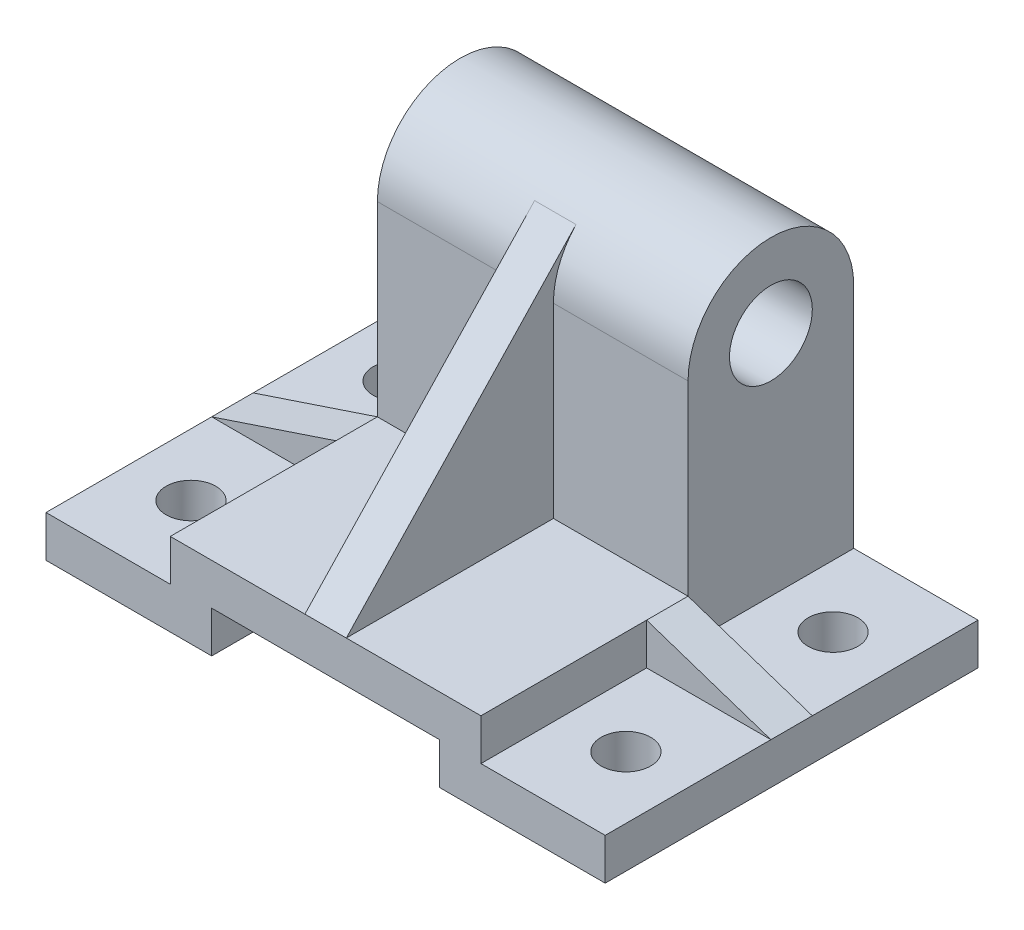
ISO-10303-21;
HEADER;
FILE_DESCRIPTION(('STEP AP214'),'2;1');
FILE_NAME('part.step','',(''),(''),'','','');
FILE_SCHEMA(('AUTOMOTIVE_DESIGN { 1 0 10303 214 1 1 1 1 }'));
ENDSEC;
DATA;
#1=APPLICATION_CONTEXT('core data for automotive mechanical design processes');
#2=APPLICATION_PROTOCOL_DEFINITION('international standard','automotive_design',2000,#1);
#3=PRODUCT_CONTEXT('',#1,'mechanical');
#4=PRODUCT('Part','Part','',(#3));
#5=PRODUCT_RELATED_PRODUCT_CATEGORY('part','',(#4));
#6=PRODUCT_DEFINITION_FORMATION('','',#4);
#7=PRODUCT_DEFINITION_CONTEXT('part definition',#1,'design');
#8=PRODUCT_DEFINITION('design','',#6,#7);
#9=PRODUCT_DEFINITION_SHAPE('','',#8);
#10=(LENGTH_UNIT() NAMED_UNIT(*) SI_UNIT(.MILLI.,.METRE.));
#11=(NAMED_UNIT(*) PLANE_ANGLE_UNIT() SI_UNIT($,.RADIAN.));
#12=(NAMED_UNIT(*) SI_UNIT($,.STERADIAN.) SOLID_ANGLE_UNIT());
#13=UNCERTAINTY_MEASURE_WITH_UNIT(LENGTH_MEASURE(1.E-05),#10,'distance_accuracy_value','');
#14=(GEOMETRIC_REPRESENTATION_CONTEXT(3) GLOBAL_UNCERTAINTY_ASSIGNED_CONTEXT((#13)) GLOBAL_UNIT_ASSIGNED_CONTEXT((#10,
#11,#12)) REPRESENTATION_CONTEXT('',''));
#15=CARTESIAN_POINT('',(0.,0.,0.));
#16=DIRECTION('',(0.,0.,1.));
#17=DIRECTION('',(1.,0.,0.));
#18=AXIS2_PLACEMENT_3D('',#15,#16,#17);
#19=CARTESIAN_POINT('',(67.5,10.,45.));
#20=DIRECTION('',(0.,-1.,0.));
#21=DIRECTION('',(1.,0.,0.));
#22=AXIS2_PLACEMENT_3D('',#19,#20,#21);
#23=PLANE('',#22);
#24=CARTESIAN_POINT('',(52.5,10.,-25.));
#25=DIRECTION('',(0.,1.,0.));
#26=DIRECTION('',(-1.,0.,0.));
#27=AXIS2_PLACEMENT_3D('',#24,#25,#26);
#28=CIRCLE('',#27,5.99999999999999);
#29=CARTESIAN_POINT('',(46.5,10.,-25.));
#30=VERTEX_POINT('',#29);
#31=EDGE_CURVE('E308',#30,#30,#28,.T.);
#32=ORIENTED_EDGE('',*,*,#31,.F.);
#33=EDGE_LOOP('',(#32));
#34=FACE_BOUND('',#33,.T.);
#35=DIRECTION('',(-1.,0.,0.));
#36=VECTOR('',#35,1.);
#37=CARTESIAN_POINT('',(67.5,10.,-5.));
#38=LINE('',#37,#36);
#39=CARTESIAN_POINT('',(67.5,10.,-4.99999999999998));
#40=VERTEX_POINT('',#39);
#41=CARTESIAN_POINT('',(37.5,10.,-4.99999999999998));
#42=VERTEX_POINT('',#41);
#43=EDGE_CURVE('E53',#40,#42,#38,.T.);
#44=ORIENTED_EDGE('',*,*,#43,.F.);
#45=DIRECTION('',(0.,0.,-1.));
#46=VECTOR('',#45,1.);
#47=CARTESIAN_POINT('',(67.5,10.,45.));
#48=LINE('',#47,#46);
#49=CARTESIAN_POINT('',(67.5,10.,-45.));
#50=VERTEX_POINT('',#49);
#51=EDGE_CURVE('E404',#40,#50,#48,.T.);
#52=ORIENTED_EDGE('',*,*,#51,.T.);
#53=DIRECTION('',(-1.,0.,0.));
#54=VECTOR('',#53,1.);
#55=CARTESIAN_POINT('',(67.5,10.,-45.));
#56=LINE('',#55,#54);
#57=CARTESIAN_POINT('',(37.5,10.,-45.));
#58=VERTEX_POINT('',#57);
#59=EDGE_CURVE('E369',#50,#58,#56,.T.);
#60=ORIENTED_EDGE('',*,*,#59,.T.);
#61=DIRECTION('',(0.,0.,-1.));
#62=VECTOR('',#61,1.);
#63=CARTESIAN_POINT('',(37.5,10.,45.));
#64=LINE('',#63,#62);
#65=EDGE_CURVE('E398',#42,#58,#64,.T.);
#66=ORIENTED_EDGE('',*,*,#65,.F.);
#67=EDGE_LOOP('',(#44,#52,#60,#66));
#68=FACE_BOUND('',#67,.T.);
#69=ADVANCED_FACE('F39',(#34,#68),#23,.F.);
#70=CARTESIAN_POINT('',(37.5,10.,45.));
#71=DIRECTION('',(-1.,0.,0.));
#72=DIRECTION('',(0.,0.,1.));
#73=AXIS2_PLACEMENT_3D('',#70,#71,#72);
#74=PLANE('',#73);
#75=CARTESIAN_POINT('',(37.5,65.,-25.));
#76=DIRECTION('',(1.,0.,0.));
#77=DIRECTION('',(0.,0.,-1.));
#78=AXIS2_PLACEMENT_3D('',#75,#76,#77);
#79=CIRCLE('',#78,10.);
#80=CARTESIAN_POINT('',(37.5,65.,-35.));
#81=VERTEX_POINT('',#80);
#82=EDGE_CURVE('E289',#81,#81,#79,.T.);
#83=ORIENTED_EDGE('',*,*,#82,.F.);
#84=EDGE_LOOP('',(#83));
#85=FACE_BOUND('',#84,.T.);
#86=DIRECTION('',(0.,1.,0.));
#87=VECTOR('',#86,1.);
#88=CARTESIAN_POINT('',(37.5,10.,-5.));
#89=LINE('',#88,#87);
#90=CARTESIAN_POINT('',(37.5,20.,-5.));
#91=VERTEX_POINT('',#90);
#92=EDGE_CURVE('E215',#42,#91,#89,.T.);
#93=ORIENTED_EDGE('',*,*,#92,.F.);
#94=ORIENTED_EDGE('',*,*,#65,.T.);
#95=DIRECTION('',(0.,1.,0.));
#96=VECTOR('',#95,1.);
#97=CARTESIAN_POINT('',(37.5,10.,-45.));
#98=LINE('',#97,#96);
#99=CARTESIAN_POINT('',(37.5,65.,-45.));
#100=VERTEX_POINT('',#99);
#101=EDGE_CURVE('E375',#58,#100,#98,.T.);
#102=ORIENTED_EDGE('',*,*,#101,.T.);
#103=CARTESIAN_POINT('',(37.5,65.,-25.));
#104=DIRECTION('',(1.,0.,0.));
#105=DIRECTION('',(0.,0.,1.));
#106=AXIS2_PLACEMENT_3D('',#103,#104,#105);
#107=CIRCLE('',#106,20.);
#108=CARTESIAN_POINT('',(37.5,65.,-5.));
#109=VERTEX_POINT('',#108);
#110=EDGE_CURVE('E214',#100,#109,#107,.T.);
#111=ORIENTED_EDGE('',*,*,#110,.T.);
#112=DIRECTION('',(0.,-1.,0.));
#113=VECTOR('',#112,1.);
#114=CARTESIAN_POINT('',(37.5,20.,-5.));
#115=LINE('',#114,#113);
#116=EDGE_CURVE('E203',#109,#91,#115,.T.);
#117=ORIENTED_EDGE('',*,*,#116,.T.);
#118=EDGE_LOOP('',(#93,#94,#102,#111,#117));
#119=FACE_BOUND('',#118,.T.);
#120=ADVANCED_FACE('F209',(#85,#119),#74,.F.);
#121=CARTESIAN_POINT('',(-37.5,20.,45.));
#122=DIRECTION('',(1.,0.,0.));
#123=DIRECTION('',(0.,0.,-1.));
#124=AXIS2_PLACEMENT_3D('',#121,#122,#123);
#125=PLANE('',#124);
#126=CARTESIAN_POINT('',(-37.5,65.,-25.));
#127=DIRECTION('',(1.,0.,0.));
#128=DIRECTION('',(0.,0.,-1.));
#129=AXIS2_PLACEMENT_3D('',#126,#127,#128);
#130=CIRCLE('',#129,10.);
#131=CARTESIAN_POINT('',(-37.5,65.,-35.));
#132=VERTEX_POINT('',#131);
#133=EDGE_CURVE('E286',#132,#132,#130,.T.);
#134=ORIENTED_EDGE('',*,*,#133,.T.);
#135=EDGE_LOOP('',(#134));
#136=FACE_BOUND('',#135,.T.);
#137=DIRECTION('',(0.,-1.,0.));
#138=VECTOR('',#137,1.);
#139=CARTESIAN_POINT('',(-37.5,20.,-5.));
#140=LINE('',#139,#138);
#141=CARTESIAN_POINT('',(-37.5,20.,-5.));
#142=VERTEX_POINT('',#141);
#143=CARTESIAN_POINT('',(-37.5,10.,-5.));
#144=VERTEX_POINT('',#143);
#145=EDGE_CURVE('E255',#142,#144,#140,.T.);
#146=ORIENTED_EDGE('',*,*,#145,.F.);
#147=DIRECTION('',(0.,-1.,0.));
#148=VECTOR('',#147,1.);
#149=CARTESIAN_POINT('',(-37.5,20.,-5.));
#150=LINE('',#149,#148);
#151=CARTESIAN_POINT('',(-37.5,65.,-5.));
#152=VERTEX_POINT('',#151);
#153=EDGE_CURVE('E296',#152,#142,#150,.T.);
#154=ORIENTED_EDGE('',*,*,#153,.F.);
#155=CARTESIAN_POINT('',(-37.5,65.,-25.));
#156=DIRECTION('',(1.,0.,0.));
#157=DIRECTION('',(0.,0.,1.));
#158=AXIS2_PLACEMENT_3D('',#155,#156,#157);
#159=CIRCLE('',#158,20.);
#160=CARTESIAN_POINT('',(-37.5,65.,-45.));
#161=VERTEX_POINT('',#160);
#162=EDGE_CURVE('E216',#161,#152,#159,.T.);
#163=ORIENTED_EDGE('',*,*,#162,.F.);
#164=DIRECTION('',(0.,-1.,0.));
#165=VECTOR('',#164,1.);
#166=CARTESIAN_POINT('',(-37.5,20.,-45.));
#167=LINE('',#166,#165);
#168=CARTESIAN_POINT('',(-37.5,10.,-45.));
#169=VERTEX_POINT('',#168);
#170=EDGE_CURVE('E372',#161,#169,#167,.T.);
#171=ORIENTED_EDGE('',*,*,#170,.T.);
#172=DIRECTION('',(0.,0.,-1.));
#173=VECTOR('',#172,1.);
#174=CARTESIAN_POINT('',(-37.5,10.,45.));
#175=LINE('',#174,#173);
#176=EDGE_CURVE('E392',#144,#169,#175,.T.);
#177=ORIENTED_EDGE('',*,*,#176,.F.);
#178=EDGE_LOOP('',(#146,#154,#163,#171,#177));
#179=FACE_BOUND('',#178,.T.);
#180=ADVANCED_FACE('F443',(#136,#179),#125,.F.);
#181=CARTESIAN_POINT('',(-37.5,10.,45.));
#182=DIRECTION('',(0.,-1.,0.));
#183=DIRECTION('',(1.,0.,0.));
#184=AXIS2_PLACEMENT_3D('',#181,#182,#183);
#185=PLANE('',#184);
#186=CARTESIAN_POINT('',(-52.5,9.99999999999999,-25.));
#187=DIRECTION('',(0.,1.,0.));
#188=DIRECTION('',(1.,0.,0.));
#189=AXIS2_PLACEMENT_3D('',#186,#187,#188);
#190=CIRCLE('',#189,5.99999999999999);
#191=CARTESIAN_POINT('',(-46.5,9.99999999999999,-25.));
#192=VERTEX_POINT('',#191);
#193=EDGE_CURVE('E309',#192,#192,#190,.T.);
#194=ORIENTED_EDGE('',*,*,#193,.F.);
#195=EDGE_LOOP('',(#194));
#196=FACE_BOUND('',#195,.T.);
#197=DIRECTION('',(-1.,0.,0.));
#198=VECTOR('',#197,1.);
#199=CARTESIAN_POINT('',(-37.5,10.,-5.));
#200=LINE('',#199,#198);
#201=CARTESIAN_POINT('',(-67.5,10.,-4.99999999999998));
#202=VERTEX_POINT('',#201);
#203=EDGE_CURVE('E248',#144,#202,#200,.T.);
#204=ORIENTED_EDGE('',*,*,#203,.F.);
#205=ORIENTED_EDGE('',*,*,#176,.T.);
#206=DIRECTION('',(-1.,0.,0.));
#207=VECTOR('',#206,1.);
#208=CARTESIAN_POINT('',(-37.5,10.,-45.));
#209=LINE('',#208,#207);
#210=CARTESIAN_POINT('',(-67.5,10.,-45.));
#211=VERTEX_POINT('',#210);
#212=EDGE_CURVE('E380',#169,#211,#209,.T.);
#213=ORIENTED_EDGE('',*,*,#212,.T.);
#214=DIRECTION('',(0.,0.,-1.));
#215=VECTOR('',#214,1.);
#216=CARTESIAN_POINT('',(-67.5,10.,45.));
#217=LINE('',#216,#215);
#218=EDGE_CURVE('E389',#202,#211,#217,.T.);
#219=ORIENTED_EDGE('',*,*,#218,.F.);
#220=EDGE_LOOP('',(#204,#205,#213,#219));
#221=FACE_BOUND('',#220,.T.);
#222=ADVANCED_FACE('F534',(#196,#221),#185,.F.);
#223=CARTESIAN_POINT('',(37.5,20.,45.));
#224=DIRECTION('',(0.,-1.,0.));
#225=DIRECTION('',(1.,0.,0.));
#226=AXIS2_PLACEMENT_3D('',#223,#224,#225);
#227=PLANE('',#226);
#228=DIRECTION('',(-1.,0.,0.));
#229=VECTOR('',#228,1.);
#230=CARTESIAN_POINT('',(37.5,20.,45.));
#231=LINE('',#230,#229);
#232=CARTESIAN_POINT('',(-5.,20.,45.));
#233=VERTEX_POINT('',#232);
#234=CARTESIAN_POINT('',(-37.5,20.,45.));
#235=VERTEX_POINT('',#234);
#236=EDGE_CURVE('E345',#233,#235,#231,.T.);
#237=ORIENTED_EDGE('',*,*,#236,.F.);
#238=DIRECTION('',(0.,0.,1.));
#239=VECTOR('',#238,1.);
#240=CARTESIAN_POINT('',(-5.,20.,45.));
#241=LINE('',#240,#239);
#242=CARTESIAN_POINT('',(-5.,20.,-5.));
#243=VERTEX_POINT('',#242);
#244=EDGE_CURVE('E279',#243,#233,#241,.T.);
#245=ORIENTED_EDGE('',*,*,#244,.F.);
#246=DIRECTION('',(1.,0.,0.));
#247=VECTOR('',#246,1.);
#248=CARTESIAN_POINT('',(-37.5,20.,-5.));
#249=LINE('',#248,#247);
#250=EDGE_CURVE('E206',#142,#243,#249,.T.);
#251=ORIENTED_EDGE('',*,*,#250,.F.);
#252=DIRECTION('',(0.,0.,1.));
#253=VECTOR('',#252,1.);
#254=CARTESIAN_POINT('',(-37.5,20.,45.));
#255=LINE('',#254,#253);
#256=CARTESIAN_POINT('',(-37.5,20.,5.));
#257=VERTEX_POINT('',#256);
#258=EDGE_CURVE('E262',#142,#257,#255,.T.);
#259=ORIENTED_EDGE('',*,*,#258,.T.);
#260=DIRECTION('',(0.,0.,-1.));
#261=VECTOR('',#260,1.);
#262=CARTESIAN_POINT('',(-37.5,20.,45.));
#263=LINE('',#262,#261);
#264=EDGE_CURVE('E397',#235,#257,#263,.T.);
#265=ORIENTED_EDGE('',*,*,#264,.F.);
#266=EDGE_LOOP('',(#237,#245,#251,#259,#265));
#267=FACE_BOUND('',#266,.T.);
#268=ADVANCED_FACE('F502',(#267),#227,.F.);
#269=CARTESIAN_POINT('',(-37.5,20.,-5.));
#270=DIRECTION('',(0.,0.,1.));
#271=DIRECTION('',(1.,0.,0.));
#272=AXIS2_PLACEMENT_3D('',#269,#270,#271);
#273=PLANE('',#272);
#274=DIRECTION('',(0.,1.,0.));
#275=VECTOR('',#274,1.);
#276=CARTESIAN_POINT('',(-5.,20.,-5.));
#277=LINE('',#276,#275);
#278=CARTESIAN_POINT('',(-5.,65.,-5.));
#279=VERTEX_POINT('',#278);
#280=EDGE_CURVE('E277',#243,#279,#277,.T.);
#281=ORIENTED_EDGE('',*,*,#280,.T.);
#282=DIRECTION('',(1.,0.,0.));
#283=VECTOR('',#282,1.);
#284=CARTESIAN_POINT('',(-37.5,65.,-5.));
#285=LINE('',#284,#283);
#286=EDGE_CURVE('E210',#152,#279,#285,.T.);
#287=ORIENTED_EDGE('',*,*,#286,.F.);
#288=ORIENTED_EDGE('',*,*,#153,.T.);
#289=ORIENTED_EDGE('',*,*,#250,.T.);
#290=EDGE_LOOP('',(#281,#287,#288,#289));
#291=FACE_BOUND('',#290,.T.);
#292=ADVANCED_FACE('F545',(#291),#273,.T.);
#293=DIRECTION('',(0.,0.,-1.));
#294=VECTOR('',#293,1.);
#295=CARTESIAN_POINT('',(37.5,20.,45.));
#296=LINE('',#295,#294);
#297=CARTESIAN_POINT('',(37.5,20.,45.));
#298=VERTEX_POINT('',#297);
#299=CARTESIAN_POINT('',(37.5,20.,5.00000000000001));
#300=VERTEX_POINT('',#299);
#301=EDGE_CURVE('E221',#298,#300,#296,.T.);
#302=ORIENTED_EDGE('',*,*,#301,.T.);
#303=DIRECTION('',(0.,0.,1.));
#304=VECTOR('',#303,1.);
#305=CARTESIAN_POINT('',(37.5,20.,45.));
#306=LINE('',#305,#304);
#307=EDGE_CURVE('E219',#300,#91,#306,.F.);
#308=ORIENTED_EDGE('',*,*,#307,.T.);
#309=CARTESIAN_POINT('',(5.,20.,-5.));
#310=VERTEX_POINT('',#309);
#311=EDGE_CURVE('E197',#310,#91,#249,.T.);
#312=ORIENTED_EDGE('',*,*,#311,.F.);
#313=DIRECTION('',(0.,0.,1.));
#314=VECTOR('',#313,1.);
#315=CARTESIAN_POINT('',(5.,20.,45.));
#316=LINE('',#315,#314);
#317=CARTESIAN_POINT('',(5.,20.,45.));
#318=VERTEX_POINT('',#317);
#319=EDGE_CURVE('E284',#310,#318,#316,.T.);
#320=ORIENTED_EDGE('',*,*,#319,.T.);
#321=EDGE_CURVE('E344',#298,#318,#231,.T.);
#322=ORIENTED_EDGE('',*,*,#321,.F.);
#323=EDGE_LOOP('',(#302,#308,#312,#320,#322));
#324=FACE_BOUND('',#323,.T.);
#325=ADVANCED_FACE('F222',(#324),#227,.F.);
#326=CARTESIAN_POINT('',(-27.5,0.,45.));
#327=DIRECTION('',(-1.,0.,0.));
#328=DIRECTION('',(0.,-1.,0.));
#329=AXIS2_PLACEMENT_3D('',#326,#327,#328);
#330=PLANE('',#329);
#331=DIRECTION('',(0.,0.,-1.));
#332=VECTOR('',#331,1.);
#333=CARTESIAN_POINT('',(-27.5,0.,45.));
#334=LINE('',#333,#332);
#335=CARTESIAN_POINT('',(-27.5,0.,45.));
#336=VERTEX_POINT('',#335);
#337=CARTESIAN_POINT('',(-27.5,0.,-45.));
#338=VERTEX_POINT('',#337);
#339=EDGE_CURVE('E353',#336,#338,#334,.T.);
#340=ORIENTED_EDGE('',*,*,#339,.T.);
#341=DIRECTION('',(0.,1.,0.));
#342=VECTOR('',#341,1.);
#343=CARTESIAN_POINT('',(-27.5,0.,-45.));
#344=LINE('',#343,#342);
#345=CARTESIAN_POINT('',(-27.5,10.,-45.));
#346=VERTEX_POINT('',#345);
#347=EDGE_CURVE('E324',#338,#346,#344,.T.);
#348=ORIENTED_EDGE('',*,*,#347,.T.);
#349=DIRECTION('',(0.,0.,-1.));
#350=VECTOR('',#349,1.);
#351=CARTESIAN_POINT('',(-27.5,10.,45.));
#352=LINE('',#351,#350);
#353=CARTESIAN_POINT('',(-27.5,10.,45.));
#354=VERTEX_POINT('',#353);
#355=EDGE_CURVE('E50',#354,#346,#352,.T.);
#356=ORIENTED_EDGE('',*,*,#355,.F.);
#357=DIRECTION('',(0.,1.,0.));
#358=VECTOR('',#357,1.);
#359=CARTESIAN_POINT('',(-27.5,0.,45.));
#360=LINE('',#359,#358);
#361=EDGE_CURVE('E326',#336,#354,#360,.T.);
#362=ORIENTED_EDGE('',*,*,#361,.F.);
#363=EDGE_LOOP('',(#340,#348,#356,#362));
#364=FACE_BOUND('',#363,.T.);
#365=ADVANCED_FACE('F41',(#364),#330,.F.);
#366=CARTESIAN_POINT('',(-27.5,10.,45.));
#367=DIRECTION('',(0.,1.,0.));
#368=DIRECTION('',(0.,0.,1.));
#369=AXIS2_PLACEMENT_3D('',#366,#367,#368);
#370=PLANE('',#369);
#371=ORIENTED_EDGE('',*,*,#355,.T.);
#372=DIRECTION('',(1.,0.,0.));
#373=VECTOR('',#372,1.);
#374=CARTESIAN_POINT('',(-27.5,10.,-45.));
#375=LINE('',#374,#373);
#376=CARTESIAN_POINT('',(27.5,10.,-45.));
#377=VERTEX_POINT('',#376);
#378=EDGE_CURVE('E360',#346,#377,#375,.T.);
#379=ORIENTED_EDGE('',*,*,#378,.T.);
#380=DIRECTION('',(0.,0.,-1.));
#381=VECTOR('',#380,1.);
#382=CARTESIAN_POINT('',(27.5,10.,45.));
#383=LINE('',#382,#381);
#384=CARTESIAN_POINT('',(27.5,10.,45.));
#385=VERTEX_POINT('',#384);
#386=EDGE_CURVE('E412',#385,#377,#383,.T.);
#387=ORIENTED_EDGE('',*,*,#386,.F.);
#388=DIRECTION('',(1.,0.,0.));
#389=VECTOR('',#388,1.);
#390=CARTESIAN_POINT('',(-27.5,10.,45.));
#391=LINE('',#390,#389);
#392=EDGE_CURVE('E328',#354,#385,#391,.T.);
#393=ORIENTED_EDGE('',*,*,#392,.F.);
#394=EDGE_LOOP('',(#371,#379,#387,#393));
#395=FACE_BOUND('',#394,.T.);
#396=ADVANCED_FACE('F528',(#395),#370,.F.);
#397=CARTESIAN_POINT('',(27.5,10.,45.));
#398=DIRECTION('',(1.,0.,0.));
#399=DIRECTION('',(0.,1.,0.));
#400=AXIS2_PLACEMENT_3D('',#397,#398,#399);
#401=PLANE('',#400);
#402=ORIENTED_EDGE('',*,*,#386,.T.);
#403=DIRECTION('',(0.,-1.,0.));
#404=VECTOR('',#403,1.);
#405=CARTESIAN_POINT('',(27.5,10.,-45.));
#406=LINE('',#405,#404);
#407=CARTESIAN_POINT('',(27.5,0.,-45.));
#408=VERTEX_POINT('',#407);
#409=EDGE_CURVE('E358',#377,#408,#406,.T.);
#410=ORIENTED_EDGE('',*,*,#409,.T.);
#411=DIRECTION('',(0.,0.,-1.));
#412=VECTOR('',#411,1.);
#413=CARTESIAN_POINT('',(27.5,0.,45.));
#414=LINE('',#413,#412);
#415=CARTESIAN_POINT('',(27.5,0.,45.));
#416=VERTEX_POINT('',#415);
#417=EDGE_CURVE('E408',#416,#408,#414,.T.);
#418=ORIENTED_EDGE('',*,*,#417,.F.);
#419=DIRECTION('',(0.,-1.,0.));
#420=VECTOR('',#419,1.);
#421=CARTESIAN_POINT('',(27.5,10.,45.));
#422=LINE('',#421,#420);
#423=EDGE_CURVE('E335',#385,#416,#422,.T.);
#424=ORIENTED_EDGE('',*,*,#423,.F.);
#425=EDGE_LOOP('',(#402,#410,#418,#424));
#426=FACE_BOUND('',#425,.T.);
#427=ADVANCED_FACE('F530',(#426),#401,.F.);
#428=CARTESIAN_POINT('',(27.5,0.,45.));
#429=DIRECTION('',(0.,1.,0.));
#430=DIRECTION('',(0.,0.,1.));
#431=AXIS2_PLACEMENT_3D('',#428,#429,#430);
#432=PLANE('',#431);
#433=CARTESIAN_POINT('',(52.5,0.,25.));
#434=DIRECTION('',(0.,1.,0.));
#435=DIRECTION('',(0.,0.,1.));
#436=AXIS2_PLACEMENT_3D('',#433,#434,#435);
#437=CIRCLE('',#436,6.);
#438=CARTESIAN_POINT('',(52.5,0.,31.));
#439=VERTEX_POINT('',#438);
#440=EDGE_CURVE('E318',#439,#439,#437,.T.);
#441=ORIENTED_EDGE('',*,*,#440,.T.);
#442=EDGE_LOOP('',(#441));
#443=FACE_BOUND('',#442,.T.);
#444=ORIENTED_EDGE('',*,*,#417,.T.);
#445=DIRECTION('',(1.,0.,0.));
#446=VECTOR('',#445,1.);
#447=CARTESIAN_POINT('',(27.5,0.,-45.));
#448=LINE('',#447,#446);
#449=CARTESIAN_POINT('',(67.5,0.,-45.));
#450=VERTEX_POINT('',#449);
#451=EDGE_CURVE('E361',#408,#450,#448,.T.);
#452=ORIENTED_EDGE('',*,*,#451,.T.);
#453=DIRECTION('',(0.,0.,-1.));
#454=VECTOR('',#453,1.);
#455=CARTESIAN_POINT('',(67.5,0.,45.));
#456=LINE('',#455,#454);
#457=CARTESIAN_POINT('',(67.5,0.,45.));
#458=VERTEX_POINT('',#457);
#459=EDGE_CURVE('E407',#458,#450,#456,.T.);
#460=ORIENTED_EDGE('',*,*,#459,.F.);
#461=DIRECTION('',(1.,0.,0.));
#462=VECTOR('',#461,1.);
#463=CARTESIAN_POINT('',(27.5,0.,45.));
#464=LINE('',#463,#462);
#465=EDGE_CURVE('E331',#416,#458,#464,.T.);
#466=ORIENTED_EDGE('',*,*,#465,.F.);
#467=EDGE_LOOP('',(#444,#452,#460,#466));
#468=FACE_BOUND('',#467,.T.);
#469=CARTESIAN_POINT('',(52.5,0.,-25.));
#470=DIRECTION('',(0.,1.,0.));
#471=DIRECTION('',(0.,0.,1.));
#472=AXIS2_PLACEMENT_3D('',#469,#470,#471);
#473=CIRCLE('',#472,5.99999999999999);
#474=CARTESIAN_POINT('',(52.5,0.,-19.));
#475=VERTEX_POINT('',#474);
#476=EDGE_CURVE('E321',#475,#475,#473,.T.);
#477=ORIENTED_EDGE('',*,*,#476,.T.);
#478=EDGE_LOOP('',(#477));
#479=FACE_BOUND('',#478,.T.);
#480=ADVANCED_FACE('F458',(#443,#468,#479),#432,.F.);
#481=CARTESIAN_POINT('',(67.5,0.,45.));
#482=DIRECTION('',(-1.,0.,0.));
#483=DIRECTION('',(0.,0.,1.));
#484=AXIS2_PLACEMENT_3D('',#481,#482,#483);
#485=PLANE('',#484);
#486=ORIENTED_EDGE('',*,*,#459,.T.);
#487=DIRECTION('',(0.,1.,0.));
#488=VECTOR('',#487,1.);
#489=CARTESIAN_POINT('',(67.5,0.,-45.));
#490=LINE('',#489,#488);
#491=EDGE_CURVE('E368',#450,#50,#490,.T.);
#492=ORIENTED_EDGE('',*,*,#491,.T.);
#493=ORIENTED_EDGE('',*,*,#51,.F.);
#494=DIRECTION('',(0.,0.,-1.));
#495=VECTOR('',#494,1.);
#496=CARTESIAN_POINT('',(67.5,10.,45.));
#497=LINE('',#496,#495);
#498=CARTESIAN_POINT('',(67.5,10.,5.00000000000001));
#499=VERTEX_POINT('',#498);
#500=EDGE_CURVE('E61',#40,#499,#497,.F.);
#501=ORIENTED_EDGE('',*,*,#500,.T.);
#502=CARTESIAN_POINT('',(67.5,10.,45.));
#503=VERTEX_POINT('',#502);
#504=EDGE_CURVE('E403',#503,#499,#48,.T.);
#505=ORIENTED_EDGE('',*,*,#504,.F.);
#506=DIRECTION('',(0.,1.,0.));
#507=VECTOR('',#506,1.);
#508=CARTESIAN_POINT('',(67.5,0.,45.));
#509=LINE('',#508,#507);
#510=EDGE_CURVE('E336',#458,#503,#509,.T.);
#511=ORIENTED_EDGE('',*,*,#510,.F.);
#512=EDGE_LOOP('',(#486,#492,#493,#501,#505,#511));
#513=FACE_BOUND('',#512,.T.);
#514=ADVANCED_FACE('F455',(#513),#485,.F.);
#515=CARTESIAN_POINT('',(52.5,10.,25.));
#516=DIRECTION('',(0.,1.,0.));
#517=DIRECTION('',(-1.,0.,0.));
#518=AXIS2_PLACEMENT_3D('',#515,#516,#517);
#519=CIRCLE('',#518,6.);
#520=CARTESIAN_POINT('',(46.5,10.,25.));
#521=VERTEX_POINT('',#520);
#522=EDGE_CURVE('E310',#521,#521,#519,.T.);
#523=ORIENTED_EDGE('',*,*,#522,.F.);
#524=EDGE_LOOP('',(#523));
#525=FACE_BOUND('',#524,.T.);
#526=ORIENTED_EDGE('',*,*,#504,.T.);
#527=DIRECTION('',(-1.,0.,0.));
#528=VECTOR('',#527,1.);
#529=CARTESIAN_POINT('',(67.5,10.,5.));
#530=LINE('',#529,#528);
#531=CARTESIAN_POINT('',(37.5,10.,5.00000000000001));
#532=VERTEX_POINT('',#531);
#533=EDGE_CURVE('E233',#499,#532,#530,.T.);
#534=ORIENTED_EDGE('',*,*,#533,.T.);
#535=CARTESIAN_POINT('',(37.5,10.,45.));
#536=VERTEX_POINT('',#535);
#537=EDGE_CURVE('E402',#536,#532,#64,.T.);
#538=ORIENTED_EDGE('',*,*,#537,.F.);
#539=DIRECTION('',(-1.,0.,0.));
#540=VECTOR('',#539,1.);
#541=CARTESIAN_POINT('',(67.5,10.,45.));
#542=LINE('',#541,#540);
#543=EDGE_CURVE('E339',#503,#536,#542,.T.);
#544=ORIENTED_EDGE('',*,*,#543,.F.);
#545=EDGE_LOOP('',(#526,#534,#538,#544));
#546=FACE_BOUND('',#545,.T.);
#547=ADVANCED_FACE('F439',(#525,#546),#23,.F.);
#548=ORIENTED_EDGE('',*,*,#537,.T.);
#549=DIRECTION('',(0.,1.,0.));
#550=VECTOR('',#549,1.);
#551=CARTESIAN_POINT('',(37.5,10.,5.));
#552=LINE('',#551,#550);
#553=EDGE_CURVE('E228',#532,#300,#552,.T.);
#554=ORIENTED_EDGE('',*,*,#553,.T.);
#555=ORIENTED_EDGE('',*,*,#301,.F.);
#556=DIRECTION('',(0.,1.,0.));
#557=VECTOR('',#556,1.);
#558=CARTESIAN_POINT('',(37.5,10.,45.));
#559=LINE('',#558,#557);
#560=EDGE_CURVE('E340',#536,#298,#559,.T.);
#561=ORIENTED_EDGE('',*,*,#560,.F.);
#562=EDGE_LOOP('',(#548,#554,#555,#561));
#563=FACE_BOUND('',#562,.T.);
#564=ADVANCED_FACE('F449',(#563),#74,.F.);
#565=ORIENTED_EDGE('',*,*,#264,.T.);
#566=DIRECTION('',(0.,-1.,0.));
#567=VECTOR('',#566,1.);
#568=CARTESIAN_POINT('',(-37.5,20.,5.));
#569=LINE('',#568,#567);
#570=CARTESIAN_POINT('',(-37.5,10.,5.));
#571=VERTEX_POINT('',#570);
#572=EDGE_CURVE('E258',#257,#571,#569,.T.);
#573=ORIENTED_EDGE('',*,*,#572,.T.);
#574=CARTESIAN_POINT('',(-37.5,10.,45.));
#575=VERTEX_POINT('',#574);
#576=EDGE_CURVE('E394',#575,#571,#175,.T.);
#577=ORIENTED_EDGE('',*,*,#576,.F.);
#578=DIRECTION('',(0.,-1.,0.));
#579=VECTOR('',#578,1.);
#580=CARTESIAN_POINT('',(-37.5,20.,45.));
#581=LINE('',#580,#579);
#582=EDGE_CURVE('E347',#235,#575,#581,.T.);
#583=ORIENTED_EDGE('',*,*,#582,.F.);
#584=EDGE_LOOP('',(#565,#573,#577,#583));
#585=FACE_BOUND('',#584,.T.);
#586=ADVANCED_FACE('F456',(#585),#125,.F.);
#587=CARTESIAN_POINT('',(-52.5,9.99999999999999,25.));
#588=DIRECTION('',(0.,1.,0.));
#589=DIRECTION('',(1.,0.,0.));
#590=AXIS2_PLACEMENT_3D('',#587,#588,#589);
#591=CIRCLE('',#590,6.);
#592=CARTESIAN_POINT('',(-46.5,9.99999999999999,25.));
#593=VERTEX_POINT('',#592);
#594=EDGE_CURVE('E302',#593,#593,#591,.T.);
#595=ORIENTED_EDGE('',*,*,#594,.F.);
#596=EDGE_LOOP('',(#595));
#597=FACE_BOUND('',#596,.T.);
#598=ORIENTED_EDGE('',*,*,#576,.T.);
#599=DIRECTION('',(-1.,0.,0.));
#600=VECTOR('',#599,1.);
#601=CARTESIAN_POINT('',(-37.5,10.,5.));
#602=LINE('',#601,#600);
#603=CARTESIAN_POINT('',(-67.5,10.,5.));
#604=VERTEX_POINT('',#603);
#605=EDGE_CURVE('E259',#571,#604,#602,.T.);
#606=ORIENTED_EDGE('',*,*,#605,.T.);
#607=CARTESIAN_POINT('',(-67.5,10.,45.));
#608=VERTEX_POINT('',#607);
#609=EDGE_CURVE('E386',#608,#604,#217,.T.);
#610=ORIENTED_EDGE('',*,*,#609,.F.);
#611=DIRECTION('',(-1.,0.,0.));
#612=VECTOR('',#611,1.);
#613=CARTESIAN_POINT('',(-37.5,10.,45.));
#614=LINE('',#613,#612);
#615=EDGE_CURVE('E346',#575,#608,#614,.T.);
#616=ORIENTED_EDGE('',*,*,#615,.F.);
#617=EDGE_LOOP('',(#598,#606,#610,#616));
#618=FACE_BOUND('',#617,.T.);
#619=ADVANCED_FACE('F506',(#597,#618),#185,.F.);
#620=CARTESIAN_POINT('',(-67.5,10.,45.));
#621=DIRECTION('',(1.,0.,0.));
#622=DIRECTION('',(0.,0.,-1.));
#623=AXIS2_PLACEMENT_3D('',#620,#621,#622);
#624=PLANE('',#623);
#625=ORIENTED_EDGE('',*,*,#609,.T.);
#626=DIRECTION('',(0.,0.,1.));
#627=VECTOR('',#626,1.);
#628=CARTESIAN_POINT('',(-67.5,10.,45.));
#629=LINE('',#628,#627);
#630=EDGE_CURVE('E265',#202,#604,#629,.T.);
#631=ORIENTED_EDGE('',*,*,#630,.F.);
#632=ORIENTED_EDGE('',*,*,#218,.T.);
#633=DIRECTION('',(0.,-1.,0.));
#634=VECTOR('',#633,1.);
#635=CARTESIAN_POINT('',(-67.5,10.,-45.));
#636=LINE('',#635,#634);
#637=CARTESIAN_POINT('',(-67.5,0.,-45.));
#638=VERTEX_POINT('',#637);
#639=EDGE_CURVE('E379',#211,#638,#636,.T.);
#640=ORIENTED_EDGE('',*,*,#639,.T.);
#641=DIRECTION('',(0.,0.,-1.));
#642=VECTOR('',#641,1.);
#643=CARTESIAN_POINT('',(-67.5,0.,45.));
#644=LINE('',#643,#642);
#645=CARTESIAN_POINT('',(-67.5,0.,45.));
#646=VERTEX_POINT('',#645);
#647=EDGE_CURVE('E387',#646,#638,#644,.T.);
#648=ORIENTED_EDGE('',*,*,#647,.F.);
#649=DIRECTION('',(0.,-1.,0.));
#650=VECTOR('',#649,1.);
#651=CARTESIAN_POINT('',(-67.5,10.,45.));
#652=LINE('',#651,#650);
#653=EDGE_CURVE('E348',#608,#646,#652,.T.);
#654=ORIENTED_EDGE('',*,*,#653,.F.);
#655=EDGE_LOOP('',(#625,#631,#632,#640,#648,#654));
#656=FACE_BOUND('',#655,.T.);
#657=ADVANCED_FACE('F513',(#656),#624,.F.);
#658=CARTESIAN_POINT('',(-67.5,0.,45.));
#659=DIRECTION('',(0.,1.,0.));
#660=DIRECTION('',(0.,0.,1.));
#661=AXIS2_PLACEMENT_3D('',#658,#659,#660);
#662=PLANE('',#661);
#663=CARTESIAN_POINT('',(-52.5,0.,25.));
#664=DIRECTION('',(0.,1.,0.));
#665=DIRECTION('',(0.,0.,1.));
#666=AXIS2_PLACEMENT_3D('',#663,#664,#665);
#667=CIRCLE('',#666,6.);
#668=CARTESIAN_POINT('',(-52.5,0.,31.));
#669=VERTEX_POINT('',#668);
#670=EDGE_CURVE('E325',#669,#669,#667,.T.);
#671=ORIENTED_EDGE('',*,*,#670,.T.);
#672=EDGE_LOOP('',(#671));
#673=FACE_BOUND('',#672,.T.);
#674=ORIENTED_EDGE('',*,*,#647,.T.);
#675=DIRECTION('',(1.,0.,0.));
#676=VECTOR('',#675,1.);
#677=CARTESIAN_POINT('',(-67.5,0.,-45.));
#678=LINE('',#677,#676);
#679=EDGE_CURVE('E329',#638,#338,#678,.T.);
#680=ORIENTED_EDGE('',*,*,#679,.T.);
#681=ORIENTED_EDGE('',*,*,#339,.F.);
#682=DIRECTION('',(1.,0.,0.));
#683=VECTOR('',#682,1.);
#684=CARTESIAN_POINT('',(-67.5,0.,45.));
#685=LINE('',#684,#683);
#686=EDGE_CURVE('E352',#646,#336,#685,.T.);
#687=ORIENTED_EDGE('',*,*,#686,.F.);
#688=EDGE_LOOP('',(#674,#680,#681,#687));
#689=FACE_BOUND('',#688,.T.);
#690=CARTESIAN_POINT('',(-52.5,0.,-25.));
#691=DIRECTION('',(0.,1.,0.));
#692=DIRECTION('',(0.,0.,1.));
#693=AXIS2_PLACEMENT_3D('',#690,#691,#692);
#694=CIRCLE('',#693,5.99999999999999);
#695=CARTESIAN_POINT('',(-52.5,0.,-19.));
#696=VERTEX_POINT('',#695);
#697=EDGE_CURVE('E320',#696,#696,#694,.T.);
#698=ORIENTED_EDGE('',*,*,#697,.T.);
#699=EDGE_LOOP('',(#698));
#700=FACE_BOUND('',#699,.T.);
#701=ADVANCED_FACE('F416',(#673,#689,#700),#662,.F.);
#702=CARTESIAN_POINT('',(0.,0.,45.));
#703=DIRECTION('',(0.,0.,-1.));
#704=DIRECTION('',(-1.,0.,0.));
#705=AXIS2_PLACEMENT_3D('',#702,#703,#704);
#706=PLANE('',#705);
#707=ORIENTED_EDGE('',*,*,#321,.T.);
#708=DIRECTION('',(1.,0.,0.));
#709=VECTOR('',#708,1.);
#710=CARTESIAN_POINT('',(0.,20.,45.));
#711=LINE('',#710,#709);
#712=EDGE_CURVE('E285',#233,#318,#711,.T.);
#713=ORIENTED_EDGE('',*,*,#712,.F.);
#714=ORIENTED_EDGE('',*,*,#236,.T.);
#715=ORIENTED_EDGE('',*,*,#582,.T.);
#716=ORIENTED_EDGE('',*,*,#615,.T.);
#717=ORIENTED_EDGE('',*,*,#653,.T.);
#718=ORIENTED_EDGE('',*,*,#686,.T.);
#719=ORIENTED_EDGE('',*,*,#361,.T.);
#720=ORIENTED_EDGE('',*,*,#392,.T.);
#721=ORIENTED_EDGE('',*,*,#423,.T.);
#722=ORIENTED_EDGE('',*,*,#465,.T.);
#723=ORIENTED_EDGE('',*,*,#510,.T.);
#724=ORIENTED_EDGE('',*,*,#543,.T.);
#725=ORIENTED_EDGE('',*,*,#560,.T.);
#726=EDGE_LOOP('',(#707,#713,#714,#715,#716,#717,#718,#719,#720,#721,#722,#723,#724,#725));
#727=FACE_BOUND('',#726,.T.);
#728=ADVANCED_FACE('F472',(#727),#706,.F.);
#729=CARTESIAN_POINT('',(0.,0.,-45.));
#730=DIRECTION('',(0.,0.,-1.));
#731=DIRECTION('',(-1.,0.,0.));
#732=AXIS2_PLACEMENT_3D('',#729,#730,#731);
#733=PLANE('',#732);
#734=ORIENTED_EDGE('',*,*,#409,.F.);
#735=ORIENTED_EDGE('',*,*,#378,.F.);
#736=ORIENTED_EDGE('',*,*,#347,.F.);
#737=ORIENTED_EDGE('',*,*,#679,.F.);
#738=ORIENTED_EDGE('',*,*,#639,.F.);
#739=ORIENTED_EDGE('',*,*,#212,.F.);
#740=ORIENTED_EDGE('',*,*,#170,.F.);
#741=DIRECTION('',(1.,0.,0.));
#742=VECTOR('',#741,1.);
#743=CARTESIAN_POINT('',(-37.5,65.,-45.));
#744=LINE('',#743,#742);
#745=EDGE_CURVE('E299',#161,#100,#744,.T.);
#746=ORIENTED_EDGE('',*,*,#745,.T.);
#747=ORIENTED_EDGE('',*,*,#101,.F.);
#748=ORIENTED_EDGE('',*,*,#59,.F.);
#749=ORIENTED_EDGE('',*,*,#491,.F.);
#750=ORIENTED_EDGE('',*,*,#451,.F.);
#751=EDGE_LOOP('',(#734,#735,#736,#737,#738,#739,#740,#746,#747,#748,#749,#750));
#752=FACE_BOUND('',#751,.T.);
#753=ADVANCED_FACE('F432',(#752),#733,.T.);
#754=CARTESIAN_POINT('',(-52.5,-30.,-25.));
#755=DIRECTION('',(0.,1.,0.));
#756=DIRECTION('',(-1.,0.,0.));
#757=AXIS2_PLACEMENT_3D('',#754,#755,#756);
#758=CYLINDRICAL_SURFACE('',#757,5.99999999999999);
#759=ORIENTED_EDGE('',*,*,#193,.T.);
#760=EDGE_LOOP('',(#759));
#761=FACE_BOUND('',#760,.T.);
#762=ORIENTED_EDGE('',*,*,#697,.F.);
#763=EDGE_LOOP('',(#762));
#764=FACE_BOUND('',#763,.T.);
#765=ADVANCED_FACE('F424',(#761,#764),#758,.F.);
#766=CARTESIAN_POINT('',(-52.5,-30.,25.));
#767=DIRECTION('',(0.,1.,0.));
#768=DIRECTION('',(-1.,0.,0.));
#769=AXIS2_PLACEMENT_3D('',#766,#767,#768);
#770=CYLINDRICAL_SURFACE('',#769,6.);
#771=ORIENTED_EDGE('',*,*,#594,.T.);
#772=EDGE_LOOP('',(#771));
#773=FACE_BOUND('',#772,.T.);
#774=ORIENTED_EDGE('',*,*,#670,.F.);
#775=EDGE_LOOP('',(#774));
#776=FACE_BOUND('',#775,.T.);
#777=ADVANCED_FACE('F423',(#773,#776),#770,.F.);
#778=CARTESIAN_POINT('',(52.5,-30.,25.));
#779=DIRECTION('',(0.,1.,0.));
#780=DIRECTION('',(-1.,0.,0.));
#781=AXIS2_PLACEMENT_3D('',#778,#779,#780);
#782=CYLINDRICAL_SURFACE('',#781,6.);
#783=ORIENTED_EDGE('',*,*,#522,.T.);
#784=EDGE_LOOP('',(#783));
#785=FACE_BOUND('',#784,.T.);
#786=ORIENTED_EDGE('',*,*,#440,.F.);
#787=EDGE_LOOP('',(#786));
#788=FACE_BOUND('',#787,.T.);
#789=ADVANCED_FACE('F421',(#785,#788),#782,.F.);
#790=CARTESIAN_POINT('',(52.5,-30.,-25.));
#791=DIRECTION('',(0.,1.,0.));
#792=DIRECTION('',(-1.,0.,0.));
#793=AXIS2_PLACEMENT_3D('',#790,#791,#792);
#794=CYLINDRICAL_SURFACE('',#793,5.99999999999999);
#795=ORIENTED_EDGE('',*,*,#31,.T.);
#796=EDGE_LOOP('',(#795));
#797=FACE_BOUND('',#796,.T.);
#798=ORIENTED_EDGE('',*,*,#476,.F.);
#799=EDGE_LOOP('',(#798));
#800=FACE_BOUND('',#799,.T.);
#801=ADVANCED_FACE('F431',(#797,#800),#794,.F.);
#802=ORIENTED_EDGE('',*,*,#311,.T.);
#803=ORIENTED_EDGE('',*,*,#116,.F.);
#804=CARTESIAN_POINT('',(5.,65.,-5.));
#805=VERTEX_POINT('',#804);
#806=EDGE_CURVE('E301',#805,#109,#285,.T.);
#807=ORIENTED_EDGE('',*,*,#806,.F.);
#808=DIRECTION('',(0.,1.,0.));
#809=VECTOR('',#808,1.);
#810=CARTESIAN_POINT('',(5.,20.,-5.));
#811=LINE('',#810,#809);
#812=EDGE_CURVE('E201',#310,#805,#811,.T.);
#813=ORIENTED_EDGE('',*,*,#812,.F.);
#814=EDGE_LOOP('',(#802,#803,#807,#813));
#815=FACE_BOUND('',#814,.T.);
#816=ADVANCED_FACE('F200',(#815),#273,.T.);
#817=CARTESIAN_POINT('',(-37.5,65.,-25.));
#818=DIRECTION('',(1.,0.,0.));
#819=DIRECTION('',(0.,0.,-1.));
#820=AXIS2_PLACEMENT_3D('',#817,#818,#819);
#821=CYLINDRICAL_SURFACE('',#820,20.);
#822=ORIENTED_EDGE('',*,*,#110,.F.);
#823=ORIENTED_EDGE('',*,*,#745,.F.);
#824=ORIENTED_EDGE('',*,*,#162,.T.);
#825=ORIENTED_EDGE('',*,*,#286,.T.);
#826=CARTESIAN_POINT('',(-5.,65.,-25.));
#827=DIRECTION('',(1.,0.,0.));
#828=DIRECTION('',(0.,0.,-1.));
#829=AXIS2_PLACEMENT_3D('',#826,#827,#828);
#830=CIRCLE('',#829,20.);
#831=CARTESIAN_POINT('',(-5.,78.7311856967256,-10.4585234806764));
#832=VERTEX_POINT('',#831);
#833=EDGE_CURVE('E271',#279,#832,#830,.F.);
#834=ORIENTED_EDGE('',*,*,#833,.T.);
#835=DIRECTION('',(1.,0.,0.));
#836=VECTOR('',#835,1.);
#837=CARTESIAN_POINT('',(-37.5,78.7311856967256,-10.4585234806764));
#838=LINE('',#837,#836);
#839=CARTESIAN_POINT('',(5.,78.7311856967256,-10.4585234806764));
#840=VERTEX_POINT('',#839);
#841=EDGE_CURVE('E11',#840,#832,#838,.F.);
#842=ORIENTED_EDGE('',*,*,#841,.F.);
#843=CARTESIAN_POINT('',(5.,65.,-25.));
#844=DIRECTION('',(1.,0.,0.));
#845=DIRECTION('',(0.,0.,-1.));
#846=AXIS2_PLACEMENT_3D('',#843,#844,#845);
#847=CIRCLE('',#846,20.);
#848=EDGE_CURVE('E278',#805,#840,#847,.F.);
#849=ORIENTED_EDGE('',*,*,#848,.F.);
#850=ORIENTED_EDGE('',*,*,#806,.T.);
#851=EDGE_LOOP('',(#822,#823,#824,#825,#834,#842,#849,#850));
#852=FACE_BOUND('',#851,.T.);
#853=ADVANCED_FACE('F490',(#852),#821,.T.);
#854=CARTESIAN_POINT('',(-37.5,65.,-25.));
#855=DIRECTION('',(1.,0.,0.));
#856=DIRECTION('',(0.,0.,-1.));
#857=AXIS2_PLACEMENT_3D('',#854,#855,#856);
#858=CYLINDRICAL_SURFACE('',#857,10.);
#859=ORIENTED_EDGE('',*,*,#82,.T.);
#860=EDGE_LOOP('',(#859));
#861=FACE_BOUND('',#860,.T.);
#862=ORIENTED_EDGE('',*,*,#133,.F.);
#863=EDGE_LOOP('',(#862));
#864=FACE_BOUND('',#863,.T.);
#865=ADVANCED_FACE('F551',(#861,#864),#858,.F.);
#866=CARTESIAN_POINT('',(5.,42.5,0.));
#867=DIRECTION('',(1.,0.,0.));
#868=DIRECTION('',(0.,0.,-1.));
#869=AXIS2_PLACEMENT_3D('',#866,#867,#868);
#870=PLANE('',#869);
#871=ORIENTED_EDGE('',*,*,#812,.T.);
#872=ORIENTED_EDGE('',*,*,#848,.T.);
#873=DIRECTION('',(0.,-0.727073825966179,0.686559284836278));
#874=VECTOR('',#873,1.);
#875=CARTESIAN_POINT('',(5.,78.7311856967256,-10.4585234806764));
#876=LINE('',#875,#874);
#877=EDGE_CURVE('E268',#840,#318,#876,.T.);
#878=ORIENTED_EDGE('',*,*,#877,.T.);
#879=ORIENTED_EDGE('',*,*,#319,.F.);
#880=EDGE_LOOP('',(#871,#872,#878,#879));
#881=FACE_BOUND('',#880,.T.);
#882=ADVANCED_FACE('F492',(#881),#870,.T.);
#883=CARTESIAN_POINT('',(-5.,42.5,0.));
#884=DIRECTION('',(1.,0.,0.));
#885=DIRECTION('',(0.,0.,-1.));
#886=AXIS2_PLACEMENT_3D('',#883,#884,#885);
#887=PLANE('',#886);
#888=ORIENTED_EDGE('',*,*,#833,.F.);
#889=ORIENTED_EDGE('',*,*,#280,.F.);
#890=ORIENTED_EDGE('',*,*,#244,.T.);
#891=DIRECTION('',(0.,-0.727073825966179,0.686559284836278));
#892=VECTOR('',#891,1.);
#893=CARTESIAN_POINT('',(-5.,78.7311856967256,-10.4585234806764));
#894=LINE('',#893,#892);
#895=EDGE_CURVE('E270',#832,#233,#894,.T.);
#896=ORIENTED_EDGE('',*,*,#895,.F.);
#897=EDGE_LOOP('',(#888,#889,#890,#896));
#898=FACE_BOUND('',#897,.T.);
#899=ADVANCED_FACE('F542',(#898),#887,.F.);
#900=CARTESIAN_POINT('',(0.,78.7311856967256,-10.4585234806764));
#901=DIRECTION('',(0.,0.686559284836279,0.727073825966179));
#902=DIRECTION('',(0.,-0.727073825966179,0.686559284836278));
#903=AXIS2_PLACEMENT_3D('',#900,#901,#902);
#904=PLANE('',#903);
#905=ORIENTED_EDGE('',*,*,#895,.T.);
#906=ORIENTED_EDGE('',*,*,#712,.T.);
#907=ORIENTED_EDGE('',*,*,#877,.F.);
#908=ORIENTED_EDGE('',*,*,#841,.T.);
#909=EDGE_LOOP('',(#905,#906,#907,#908));
#910=FACE_BOUND('',#909,.T.);
#911=ADVANCED_FACE('F494',(#910),#904,.T.);
#912=CARTESIAN_POINT('',(-37.5,20.,0.));
#913=DIRECTION('',(-0.316227766016838,0.948683298050514,0.));
#914=DIRECTION('',(-0.948683298050514,-0.316227766016838,0.));
#915=AXIS2_PLACEMENT_3D('',#912,#913,#914);
#916=PLANE('',#915);
#917=ORIENTED_EDGE('',*,*,#258,.F.);
#918=DIRECTION('',(-0.948683298050514,-0.316227766016838,0.));
#919=VECTOR('',#918,1.);
#920=CARTESIAN_POINT('',(-37.5,20.,-5.));
#921=LINE('',#920,#919);
#922=EDGE_CURVE('E247',#142,#202,#921,.T.);
#923=ORIENTED_EDGE('',*,*,#922,.T.);
#924=ORIENTED_EDGE('',*,*,#630,.T.);
#925=DIRECTION('',(-0.948683298050514,-0.316227766016838,0.));
#926=VECTOR('',#925,1.);
#927=CARTESIAN_POINT('',(-37.5,20.,5.));
#928=LINE('',#927,#926);
#929=EDGE_CURVE('E250',#257,#604,#928,.T.);
#930=ORIENTED_EDGE('',*,*,#929,.F.);
#931=EDGE_LOOP('',(#917,#923,#924,#930));
#932=FACE_BOUND('',#931,.T.);
#933=ADVANCED_FACE('F555',(#932),#916,.T.);
#934=CARTESIAN_POINT('',(0.,42.5,5.));
#935=DIRECTION('',(0.,0.,1.));
#936=DIRECTION('',(1.,0.,0.));
#937=AXIS2_PLACEMENT_3D('',#934,#935,#936);
#938=PLANE('',#937);
#939=ORIENTED_EDGE('',*,*,#605,.F.);
#940=ORIENTED_EDGE('',*,*,#572,.F.);
#941=ORIENTED_EDGE('',*,*,#929,.T.);
#942=EDGE_LOOP('',(#939,#940,#941));
#943=FACE_BOUND('',#942,.T.);
#944=ADVANCED_FACE('F700',(#943),#938,.T.);
#945=CARTESIAN_POINT('',(0.,42.5,-5.));
#946=DIRECTION('',(0.,0.,1.));
#947=DIRECTION('',(1.,0.,0.));
#948=AXIS2_PLACEMENT_3D('',#945,#946,#947);
#949=PLANE('',#948);
#950=ORIENTED_EDGE('',*,*,#922,.F.);
#951=ORIENTED_EDGE('',*,*,#145,.T.);
#952=ORIENTED_EDGE('',*,*,#203,.T.);
#953=EDGE_LOOP('',(#950,#951,#952));
#954=FACE_BOUND('',#953,.T.);
#955=ADVANCED_FACE('F706',(#954),#949,.F.);
#956=CARTESIAN_POINT('',(37.5,20.,0.));
#957=DIRECTION('',(-0.316227766016838,-0.948683298050514,0.));
#958=DIRECTION('',(0.948683298050514,-0.316227766016838,0.));
#959=AXIS2_PLACEMENT_3D('',#956,#957,#958);
#960=PLANE('',#959);
#961=ORIENTED_EDGE('',*,*,#500,.F.);
#962=DIRECTION('',(0.948683298050514,-0.316227766016838,0.));
#963=VECTOR('',#962,1.);
#964=CARTESIAN_POINT('',(37.5,20.,-5.));
#965=LINE('',#964,#963);
#966=EDGE_CURVE('E231',#91,#40,#965,.T.);
#967=ORIENTED_EDGE('',*,*,#966,.F.);
#968=ORIENTED_EDGE('',*,*,#307,.F.);
#969=DIRECTION('',(0.948683298050514,-0.316227766016838,0.));
#970=VECTOR('',#969,1.);
#971=CARTESIAN_POINT('',(37.5,20.,5.));
#972=LINE('',#971,#970);
#973=EDGE_CURVE('E236',#300,#499,#972,.T.);
#974=ORIENTED_EDGE('',*,*,#973,.T.);
#975=EDGE_LOOP('',(#961,#967,#968,#974));
#976=FACE_BOUND('',#975,.T.);
#977=ADVANCED_FACE('F240',(#976),#960,.F.);
#978=CARTESIAN_POINT('',(0.,42.5,5.));
#979=DIRECTION('',(0.,0.,1.));
#980=DIRECTION('',(1.,0.,0.));
#981=AXIS2_PLACEMENT_3D('',#978,#979,#980);
#982=PLANE('',#981);
#983=ORIENTED_EDGE('',*,*,#553,.F.);
#984=ORIENTED_EDGE('',*,*,#533,.F.);
#985=ORIENTED_EDGE('',*,*,#973,.F.);
#986=EDGE_LOOP('',(#983,#984,#985));
#987=FACE_BOUND('',#986,.T.);
#988=ADVANCED_FACE('F466',(#987),#982,.T.);
#989=CARTESIAN_POINT('',(0.,42.5,-5.));
#990=DIRECTION('',(0.,0.,1.));
#991=DIRECTION('',(1.,0.,0.));
#992=AXIS2_PLACEMENT_3D('',#989,#990,#991);
#993=PLANE('',#992);
#994=ORIENTED_EDGE('',*,*,#43,.T.);
#995=ORIENTED_EDGE('',*,*,#92,.T.);
#996=ORIENTED_EDGE('',*,*,#966,.T.);
#997=EDGE_LOOP('',(#994,#995,#996));
#998=FACE_BOUND('',#997,.T.);
#999=ADVANCED_FACE('F234',(#998),#993,.F.);
#1000=CLOSED_SHELL('',(#69,#120,#180,#222,#268,#292,#325,#365,#396,#427,#480,#514,#547,#564,
#586,#619,#657,#701,#728,#753,#765,#777,#789,#801,#816,#853,#865,#882,#899,#911,#933,#944,#955,
#977,#988,#999));
#1001=MANIFOLD_SOLID_BREP('B2',#1000);
#1002=ADVANCED_BREP_SHAPE_REPRESENTATION('',(#18,#1001),#14);
#1003=SHAPE_DEFINITION_REPRESENTATION(#9,#1002);
ENDSEC;
END-ISO-10303-21;
